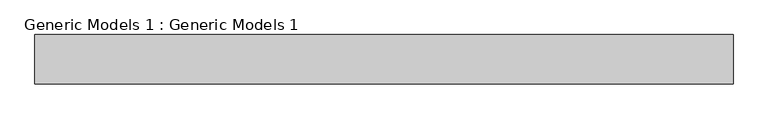
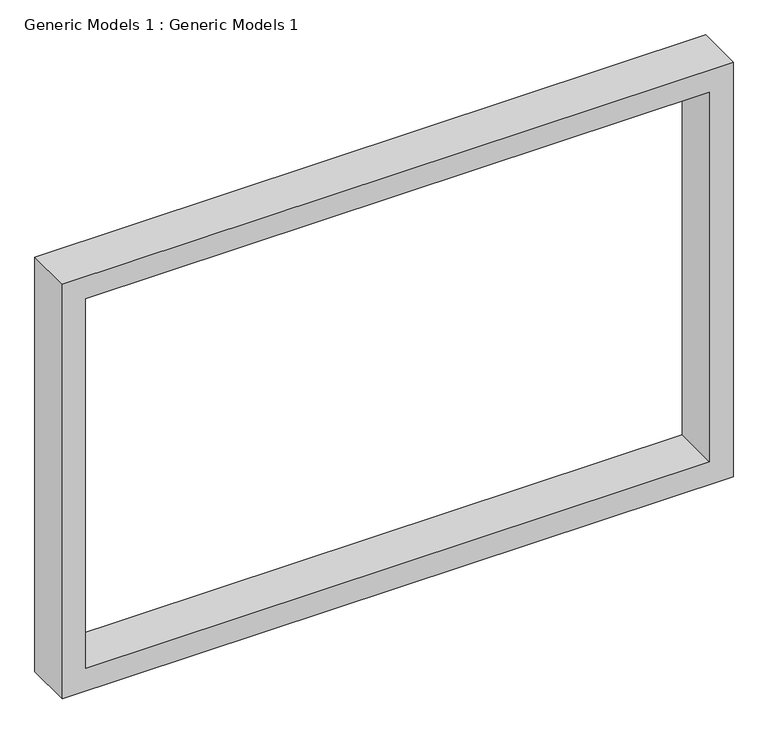
"""IFC4 building model written with IfcOpenShell, lengths in millimetres: proxy geometry, Generic Models 1 : Generic Models 1."""

from ifc_helpers import new_model, si_unit, frame, origin, place, context, project, spatial, polyline, outline, extrude, source, transform, mapped, element, save


def generic_models_1_generic_models_1_e6ddf01a(model_context):
    return source(origin(), model_context, "Body", "SweptSolid", [
        extrude(outline(polyline([(5689.0, -995.273248), (5689.0, -3157.673248), (4276.6, -3157.673248), (4276.6, -995.273248), (5689.0, -995.273248)]), holes=[polyline([(5612.8, -1071.473248), (4352.8, -1071.473248), (4352.8, -3081.473248), (5612.8, -3081.473248), (5612.8, -1071.473248)])]), frame((0.0, -3924.8866303, 0.0), z_axis=(0.0, 1.0, 0.0), x_axis=(0.0, 0.0, 1.0)), (0.0, 0.0, 1.0), 152.4),
    ])


if __name__ == "__main__":
    model = new_model("IFC4")
    model_context = context("Model", 3, world=origin())
    ifc_project = project(units=[si_unit("LENGTHUNIT", "METRE", prefix="MILLI")], contexts=[model_context])
    site = spatial("IfcSite", under=ifc_project)
    building = spatial("IfcBuilding", under=site)
    placement = place(None, origin())
    generic_models_1_generic_models_1_shape = generic_models_1_generic_models_1_e6ddf01a(model_context)
    element("IfcBuildingElementProxy", 1, Name="Generic Models 1 : Generic Models 1", ObjectType="Generic Models 1 : Generic Models 1", at=placement, inside=building, context=model_context, shape_type="MappedRepresentation", body=[
        mapped(generic_models_1_generic_models_1_shape, transform((0.0, 0.0, 0.0), x_axis=(1.0, 0.0, 0.0), y_axis=(0.0, 1.0, 0.0), z_axis=(0.0, 0.0, 1.0))),
    ])
    save(model, "model.ifc")

# Revit data of these elements
# Element 1 (IfcBuildingElementProxy, "Generic Models 1 : Generic Models 1")
#   Materials on its faces: "BLACK FRAMING 6\""
# Materials
#   "BLACK FRAMING 6\"": class "Generic", colour RGB 120 120 120, transparency 0, Cost = 0
